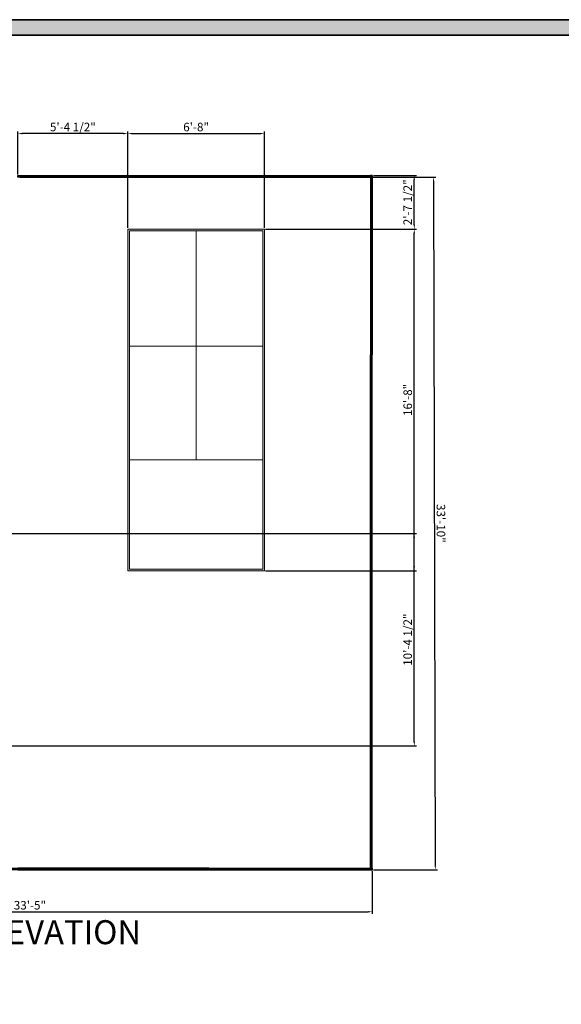
# Model space of a CAD drawing. Units: inches. Extents: x 1804 to 3296, y 909 to 2477.
# Tile 28 of 31: x 2117 to 2434, y 1900 to 2477. Entities that reach past the tile are written whole.
import ezdxf

# ---------------------------------------------------------------- set-up
doc = ezdxf.new("R2010")
doc.units = ezdxf.units.IN
for name, color, linetype, lineweight in [('A-ANNO-DIMS', 2, 'Continuous', 18), ('A-ANNO-TTLB', 156, 'Continuous', 35), ('A-ELEV-PATT', 85, 'Continuous', 13), ('A-WALL-PATT', 10, 'Continuous', 13), ('ELE', 210, 'Continuous', 30), ('TEXT', 190, 'Continuous', 18), ('WIND', 130, 'Continuous', 18)]:
    doc.layers.add(name, color=color, linetype=linetype, lineweight=lineweight)
doc.styles.get("Standard").update_dxf_attribs({"font": 'arial.ttf'})
doc.dimstyles.new('ISO-25', dxfattribs={"dimtxt": 5, "dimasz": 2.5, "dimexe": 1.25, "dimexo": 0.625, "dimtad": 1, "dimdec": 0, "dimlunit": 4, "dimtxsty": 'Standard', "dimcen": 2.5, "dimadec": 0, "dimazin": 0, "dimtfac": 1, "dimtdec": 0, "dimtmove": 0, "dimatfit": 3, "dimfxl": 1, "dimarcsym": 0})

# ---------------------------------------------------------------- blocks, each defined once
blk = doc.blocks.new('*D32')
at = {"layer": 'A-ANNO-DIMS', "color": 0, "lineweight": -2, "transparency": 16777216}
for p, q in [((2322.75, 2384.31), (2360.22, 2384.4)), ((2358.98, 2381.9), (2359.97, 1981.38)), ((2323.75, 1978.79), (2361.22, 1978.88))]:
    blk.add_line(p, q, dxfattribs=at)
at = {"layer": 'A-ANNO-DIMS', "color": 0, "lineweight": 100, "transparency": 16777216}
for points in [[(2359.4, 2381.9), (2358.56, 2381.9), (2358.97, 2384.4)], [(2360.38, 1981.38), (2359.55, 1981.38), (2359.97, 1978.88)]]:
    blk.add_solid(points, dxfattribs=at)
at = {"layer": 'Defpoints', "color": 0, "lineweight": 100, "transparency": 16777216}
for p in [(2322.12, 2384.31), (2323.12, 1978.79), (2359.97, 1978.88)]:
    blk.add_point(p, dxfattribs=at)
at = {"layer": 'A-ANNO-DIMS', "color": 0, "transparency": 16777216, "insert": (2362.65, 2181.65), "char_height": 5, "attachment_point": 5, "rotation": 270.14129}
blk.add_mtext('33\'-10"', dxfattribs=at)
blk = doc.blocks.new('*D75')
at = {"layer": 'A-ANNO-DIMS', "color": 0, "lineweight": -2, "transparency": 16777216}
for p, q in [((1922.17, 1978.16), (1922.17, 1952.99)), ((2323.12, 1978.16), (2323.12, 1952.99)), ((1924.67, 1954.24), (2320.62, 1954.24))]:
    blk.add_line(p, q, dxfattribs=at)
at = {"layer": 'A-ANNO-DIMS', "color": 0, "lineweight": 100, "transparency": 16777216}
for points in [[(1924.67, 1954.65), (1924.67, 1953.82), (1922.17, 1954.24)], [(2320.62, 1954.65), (2320.62, 1953.82), (2323.12, 1954.24)]]:
    blk.add_solid(points, dxfattribs=at)
at = {"layer": 'Defpoints', "color": 0, "lineweight": 100, "transparency": 16777216}
for p in [(1922.17, 1978.79), (2323.12, 1978.79), (2323.12, 1954.24)]:
    blk.add_point(p, dxfattribs=at)
at = {"layer": 'A-ANNO-DIMS', "color": 0, "transparency": 16777216, "insert": (2122.65, 1957.42), "char_height": 5, "attachment_point": 5}
blk.add_mtext('33\'-5"', dxfattribs=at)
blk = doc.blocks.new('*D83')
at = {"layer": 'A-ANNO-DIMS', "color": 0, "lineweight": -2, "transparency": 16777216}
for p, q in [((2054.05, 2175.81), (2348.92, 2175.81)), ((2347.67, 2053.81), (2347.67, 2173.31)), ((2054.05, 2051.31), (2348.92, 2051.31))]:
    blk.add_line(p, q, dxfattribs=at)
at = {"layer": 'A-ANNO-DIMS', "color": 0, "lineweight": 100, "transparency": 16777216}
for points in [[(2347.26, 2173.31), (2348.09, 2173.31), (2347.67, 2175.81)], [(2347.26, 2053.81), (2348.09, 2053.81), (2347.67, 2051.31)]]:
    blk.add_solid(points, dxfattribs=at)
at = {"layer": 'Defpoints', "color": 0, "lineweight": 100, "transparency": 16777216}
for p in [(2053.42, 2175.81), (2347.67, 2175.81), (2053.42, 2051.31)]:
    blk.add_point(p, dxfattribs=at)
at = {"layer": 'A-ANNO-DIMS', "color": 0, "transparency": 16777216, "insert": (2344.46, 2113.56), "char_height": 5, "attachment_point": 5, "rotation": 90}
blk.add_mtext('10\'-4 1/2"', dxfattribs=at)
blk = doc.blocks.new('*D84')
at = {"layer": 'A-ANNO-DIMS', "color": 0, "lineweight": -2, "transparency": 16777216}
for p, q in [((2179.93, 2354.6), (2179.93, 2411.11)), ((2182.43, 2409.86), (2257.48, 2409.86)), ((2259.98, 2354.6), (2259.98, 2411.11))]:
    blk.add_line(p, q, dxfattribs=at)
at = {"layer": 'A-ANNO-DIMS', "color": 0, "lineweight": 100, "transparency": 16777216}
for points in [[(2182.43, 2410.28), (2182.43, 2409.44), (2179.93, 2409.86)], [(2257.48, 2410.28), (2257.48, 2409.44), (2259.98, 2409.86)]]:
    blk.add_solid(points, dxfattribs=at)
at = {"layer": 'Defpoints', "color": 0, "lineweight": 100, "transparency": 16777216}
for p in [(2259.98, 2409.86), (2179.93, 2353.97), (2259.98, 2353.97)]:
    blk.add_point(p, dxfattribs=at)
at = {"layer": 'A-ANNO-DIMS', "color": 0, "transparency": 16777216, "insert": (2219.96, 2413.04), "char_height": 5, "attachment_point": 5}
blk.add_mtext('6\'-8"', dxfattribs=at)
blk = doc.blocks.new('*D85')
at = {"layer": 'A-ANNO-DIMS', "color": 0, "lineweight": -2, "transparency": 16777216}
for p, q in [((2260.61, 2353.97), (2348.92, 2353.97)), ((2347.67, 2156.42), (2347.67, 2351.47)), ((2260.61, 2153.92), (2348.92, 2153.92))]:
    blk.add_line(p, q, dxfattribs=at)
at = {"layer": 'A-ANNO-DIMS', "color": 0, "lineweight": 100, "transparency": 16777216}
for points in [[(2347.26, 2351.47), (2348.09, 2351.47), (2347.67, 2353.97)], [(2347.26, 2156.42), (2348.09, 2156.42), (2347.67, 2153.92)]]:
    blk.add_solid(points, dxfattribs=at)
at = {"layer": 'Defpoints', "color": 0, "lineweight": 100, "transparency": 16777216}
for p in [(2259.98, 2353.97), (2347.67, 2353.97), (2259.98, 2153.92)]:
    blk.add_point(p, dxfattribs=at)
at = {"layer": 'A-ANNO-DIMS', "color": 0, "transparency": 16777216, "insert": (2344.5, 2253.94), "char_height": 5, "attachment_point": 5, "rotation": 90}
blk.add_mtext('16\'-8"', dxfattribs=at)
blk = doc.blocks.new('*D86')
at = {"layer": 'A-ANNO-DIMS', "color": 0, "lineweight": -2, "transparency": 16777216}
for p, q in [((2115.67, 2385.93), (2115.67, 2411.11)), ((2177.43, 2409.86), (2118.17, 2409.86)), ((2179.93, 2354.6), (2179.93, 2411.11))]:
    blk.add_line(p, q, dxfattribs=at)
at = {"layer": 'A-ANNO-DIMS', "color": 0, "lineweight": 100, "transparency": 16777216}
for points in [[(2118.17, 2410.28), (2118.17, 2409.44), (2115.67, 2409.86)], [(2177.43, 2410.28), (2177.43, 2409.44), (2179.93, 2409.86)]]:
    blk.add_solid(points, dxfattribs=at)
at = {"layer": 'Defpoints', "color": 0, "lineweight": 100, "transparency": 16777216}
for p in [(2115.67, 2409.86), (2115.67, 2385.31), (2179.93, 2353.97)]:
    blk.add_point(p, dxfattribs=at)
at = {"layer": 'A-ANNO-DIMS', "color": 0, "transparency": 16777216, "insert": (2147.8, 2413.07), "char_height": 5, "attachment_point": 5}
blk.add_mtext('5\'-4 1/2"', dxfattribs=at)
blk = doc.blocks.new('*D87')
at = {"layer": 'A-ANNO-DIMS', "color": 0, "lineweight": -2, "transparency": 16777216}
for p, q in [((2323.75, 2385.31), (2348.92, 2385.31)), ((2347.67, 2356.47), (2347.67, 2382.81)), ((2260.61, 2353.97), (2348.92, 2353.97))]:
    blk.add_line(p, q, dxfattribs=at)
at = {"layer": 'A-ANNO-DIMS', "color": 0, "lineweight": 100, "transparency": 16777216}
for points in [[(2347.26, 2382.81), (2348.09, 2382.81), (2347.67, 2385.31)], [(2347.26, 2356.47), (2348.09, 2356.47), (2347.67, 2353.97)]]:
    blk.add_solid(points, dxfattribs=at)
at = {"layer": 'Defpoints', "color": 0, "lineweight": 100, "transparency": 16777216}
for p in [(2323.12, 2385.31), (2347.67, 2385.31), (2259.98, 2353.97)]:
    blk.add_point(p, dxfattribs=at)
at = {"layer": 'A-ANNO-DIMS', "color": 0, "transparency": 16777216, "insert": (2344.46, 2369.64), "char_height": 5, "attachment_point": 5, "rotation": 90}
blk.add_mtext('2\'-7 1/2"', dxfattribs=at)

msp = doc.modelspace()

# ---------------------------------------------------------------- hatches: boundary and pattern name
at = {"layer": 'A-ANNO-TTLB'}
h = msp.add_hatch(color=256, dxfattribs=at)
h.dxf.hatch_style = 1
h.paths.add_polyline_path([(3294.53, 2476.54), (1803.79, 2476.54), (1805.43, 909.47), (3296.17, 909.47)])
h.paths.add_polyline_path([(1811, 914.33), (1812.79, 2467.54), (3285.53, 2467.54), (3283.74, 914.33)], flags=16)
h.paths.add_polyline_path([(1925.58, 1062.77), (1925.58, 1138.07), (1925.58, 1539.88), (1925.58, 1793.38), (1925.58, 1830.04), (2325.54, 1830.04), (2325.54, 1793.38), (2325.54, 1586.42), (2325.54, 1138.07), (2325.54, 1062.77)], flags=0)
h.paths.add_polyline_path([(1997.22, 1029.4), (2008.85, 1037.96), (2008.85, 1020.84)], flags=0)
h.paths.add_polyline_path([(1934.58, 1138.07), (1934.58, 1147.07), (2078.77, 1147.07), (2078.77, 1138.07), (2060.94, 1138.07)], flags=0)
h.paths.add_polyline_path([(1944.35, 1138.07), (1944.35, 1147.07), (2056.05, 1147.07), (2056.05, 1138.07)], flags=0)
h.paths.add_polyline_path([(2222.24, 1037.96), (2233.87, 1029.4), (2222.24, 1020.84)], flags=0)
h.paths.add_polyline_path([(2061.94, 1139.07), (2061.94, 1146.07), (2077.77, 1146.07), (2077.77, 1139.07)], flags=0)
h.paths.add_polyline_path([(2149.58, 1138.07), (2149.58, 1269.44), (2158.58, 1269.44), (2158.58, 1326.69), (2149.58, 1326.69), (2149.58, 1340.94), (2139.6, 1340.94), (2139.6, 1434.25), (2149.58, 1434.25), (2149.58, 1447.36), (2158.58, 1447.36), (2158.58, 1423.87), (2158.58, 1408.06), (2198.46, 1408.06), (2198.46, 1412.56), (2282.65, 1412.56), (2282.65, 1465.94), (2316.54, 1465.94), (2316.54, 1590.92), (2192.86, 1590.92), (2192.86, 1595.3), (2291.17, 1595.3), (2291.17, 1590.92), (2316.54, 1590.92), (2316.54, 1784.38), (2300.24, 1784.38), (2300.24, 1757.47), (2268, 1757.47), (2268, 1681.04), (2180.87, 1681.04), (2180.87, 1757.47), (2148.63, 1757.47), (2148.63, 1784.38), (2119.08, 1784.38), (2119.08, 1585.58), (2114.58, 1585.58), (2114.58, 1784.38), (2064.11, 1784.38), (2046.28, 1784.38), (2046.28, 1760.38), (1958.58, 1760.38), (1958.58, 1664.38), (1934.58, 1664.38), (1934.58, 1784.38), (1934.58, 1793.38), (2046.28, 1793.38), (2064.11, 1793.38), (2119.08, 1793.38), (2230.78, 1793.38), (2230.78, 1784.38), (2268, 1784.38), (2300.24, 1784.38), (2316.54, 1784.38), (2316.54, 1590.92), (2316.54, 1373.73), (2316.54, 1138.07)], flags=0)
h.paths.add_polyline_path([(2209.19, 1166.63), (2209.19, 1175.63), (2158.58, 1175.63), (2209.19, 1223.63), (2209.19, 1231.63), (2183.88, 1231.63), (2183.88, 1301.66), (2242.59, 1301.66), (2242.59, 1326.69), (2316.54, 1326.69), (2272.59, 1271.63), (2272.59, 1223.63), (2316.54, 1175.63), (2272.59, 1175.63), (2272.59, 1166.63)], flags=0)
h.paths.add_polyline_path([(1947.77, 1345.22), (1947.77, 1457.48), (1991.2, 1457.48), (1991.2, 1451.7), (1991.2, 1352.18), (1991.2, 1345.22)], flags=0)
h.paths.add_polyline_path([(2209.19, 1271.63), (2262.59, 1271.63), (2262.59, 1311.85), (2272.59, 1301.66), (2272.59, 1271.63), (2269.92, 1269.63), (2270.59, 1269.63), (2270.59, 1225.63), (2211.19, 1225.63), (2211.19, 1269.63), (2211.86, 1269.63)], flags=0)
h.paths.add_polyline_path([(2000.34, 1378.21), (2000.34, 1429.71), (2025.22, 1429.71), (2025.22, 1378.21)], flags=0)
h.paths.add_polyline_path([(2001.34, 1379.21), (2001.34, 1428.71), (2024.22, 1428.71), (2024.22, 1379.21)], flags=0)
h.paths.add_polyline_path([(2012.34, 1390.21), (2012.34, 1417.71), (2013.22, 1417.71), (2013.22, 1390.21)], flags=0)
h.paths.add_polyline_path([(2237.56, 1331.19), (2237.56, 1340.18), (2238.62, 1340.18), (2238.62, 1386.84), (2241.04, 1386.84), (2242.06, 1386.84), (2242.06, 1408.06), (2316.54, 1331.19)], flags=0)
h.paths.add_polyline_path([(1953.73, 1464.35), (1953.73, 1498.59), (1981.74, 1498.59), (1981.74, 1464.35)], flags=0)
h.paths.add_polyline_path([(1987.63, 1462.08), (1987.63, 1500.95), (2104.07, 1500.95), (2104.07, 1462.08), (2099.27, 1462.08), (1993.6, 1462.08)], flags=0)
h.paths.add_polyline_path([(1956.06, 1481.47, -1), (1979.41, 1481.47, -1)], flags=0)
edge = h.paths.add_edge_path(flags=0)
edge.add_ellipse((2299.53, 1438.37), major_axis=(0.31, 21.36), ratio=0.670333, start_angle=0, end_angle=360)
h.paths.add_polyline_path([(2297.39, 1438.37, -1), (2301.67, 1438.37, -1)], flags=0)
h.paths.add_polyline_path([(2591.54, 1163.23), (2591.54, 1179.38), (2591.54, 1379.68), (2591.54, 1395.84), (2734.5, 1395.84), (2734.5, 1379.68), (2734.5, 1179.38), (2734.5, 1163.23)], flags=0)
h.paths.add_polyline_path([(2592.54, 1164.23), (2592.54, 1166.23), (2733.5, 1166.23), (2733.5, 1164.23)], flags=0)
h.paths.add_polyline_path([(2592.54, 1180.38), (2592.54, 1378.68), (2733.5, 1378.68), (2733.5, 1180.38)], flags=0)
h.paths.add_polyline_path([(2593.54, 1181.38), (2593.54, 1377.68), (2732.5, 1377.68), (2732.5, 1181.38)], flags=0)
h.paths.add_polyline_path([(2594.54, 1182.38), (2594.54, 1376.68), (2731.5, 1376.68), (2731.5, 1182.38)], flags=0)
h.paths.add_polyline_path([(1936.95, 1697.46), (1936.95, 1736.46), (1955.41, 1736.46), (1955.41, 1697.46)], flags=0)
h.paths.add_polyline_path([(1938.48, 1718.36), (1938.48, 1734.92), (1953.65, 1734.92), (1953.65, 1718.36)], flags=0)
h.paths.add_polyline_path([(1944.75, 1726.64, -1), (1947.37, 1726.64, -1)], flags=0)
h.paths.add_polyline_path([(2592.54, 1394.84), (2733.5, 1394.84), (2733.5, 1392.84), (2592.54, 1392.84)], flags=0)
h.paths.add_polyline_path([(1976.61, 1762.5), (1976.61, 1781.44), (2012.79, 1781.44), (2012.79, 1762.5)], flags=0)
h.paths.add_polyline_path([(1979.57, 1771.97, -1), (1991.39, 1771.97, -1)], flags=0)
h.paths.add_polyline_path([(1995.36, 1771.97, -1), (2007.18, 1771.97, -1)], flags=0)
h.paths.add_polyline_path([(2251.51, 1744.53), (2268, 1730.05), (2251.51, 1730.05)], flags=0)
h.paths.add_polyline_path([(2047.28, 1785.38), (2047.28, 1792.38), (2063.11, 1792.38), (2063.11, 1785.38)], flags=0)
h.paths.add_polyline_path([(2155.08, 1770.92, -1), (2174.42, 1770.92, -1)], flags=0)
h.paths.add_polyline_path([(2188.59, 1758.27), (2188.59, 1772.81), (2222.3, 1772.81), (2222.3, 1758.27)], flags=0)
h.paths.add_polyline_path([(2223.97, 1758.27), (2223.97, 1772.81), (2257.68, 1772.81), (2257.68, 1758.27)], flags=0)
h.paths.add_polyline_path([(2274.45, 1770.92, -1), (2293.8, 1770.92, -1)], flags=0)
h.paths.add_polyline_path([(2591.54, 1582.09), (2591.54, 1782.39), (2734.5, 1782.39), (2734.5, 1582.09)], flags=0)
h.paths.add_polyline_path([(2592.54, 1583.09), (2592.54, 1781.39), (2733.5, 1781.39), (2733.5, 1583.09)], flags=0)
h.paths.add_polyline_path([(2593.54, 1584.09), (2593.54, 1780.39), (2732.5, 1780.39), (2732.5, 1584.09)], flags=0)
h.paths.add_polyline_path([(2594.54, 1585.09), (2594.54, 1779.39), (2731.5, 1779.39), (2731.5, 1585.09)], flags=0)
h.paths.add_polyline_path([(1922.17, 1978.79), (1922.17, 2295.08), (1922.17, 2296.08), (2115.67, 2296.08), (2115.67, 2384.31), (2115.67, 2385.31), (2322.12, 2385.31), (2323.12, 2385.31), (2323.12, 1979.79), (2323.12, 1978.79), (1923.17, 1978.79)], flags=0)
h.paths.add_polyline_path([(1922.17, 1978.79), (1922.17, 2051.31), (1922.17, 2214.86), (1922.17, 2296.08), (2115.67, 2296.08), (2115.67, 2385.31), (2323.12, 2385.31), (2323.12, 2280.42), (2323.12, 1978.79), (2115.67, 1978.79)], flags=0)
h.paths.add_polyline_path([(1923.17, 1979.79), (1923.17, 2050.31), (2115.67, 2050.31), (2115.67, 2051.31), (1923.17, 2051.31), (1923.17, 2213.86), (1923.17, 2214.86), (1923.17, 2295.08), (1990.02, 2295.08), (1990.02, 2214.86), (1991.02, 2214.86), (1991.02, 2295.08), (2115.67, 2295.08), (2115.67, 1979.79), (2116.67, 1979.79), (2116.67, 2304.18), (2116.67, 2384.31), (2322.12, 2384.31), (2322.12, 2280.42), (2322.12, 1979.79), (2115.67, 1979.79)], flags=0)
h.paths.add_polyline_path([(2972.46, 1192.5), (2972.46, 1196.92), (2995.47, 1196.92), (2995.47, 1255.47), (2995.09, 1255.47), (2987.42, 1249.39), (2980.08, 1255.47), (2978.05, 1255.47), (2978.05, 1257.24), (2995.47, 1257.24), (2995.47, 1261.58), (3015.37, 1261.58), (3015.37, 1333.28), (3015.37, 1414.4), (3032.82, 1414.4), (3032.82, 1333.28), (3032.82, 1261.58), (3052.66, 1261.58), (3052.66, 1255.47), (3079.86, 1255.47), (3078.72, 1254.57), (3081.47, 1252.29), (3078.56, 1249.99), (3075.81, 1252.26), (3072.57, 1249.69), (3070.36, 1251.52), (3067.67, 1249.39), (3060.34, 1255.47), (3052.66, 1255.47), (3052.66, 1196.92), (3054.58, 1196.92), (3074, 1196.92), (3074, 1192.5), (3052.66, 1192.5), (2995.47, 1192.5)], flags=0)
h.paths.add_polyline_path([(2490.75, 1979.27), (2490.75, 1980.27), (2596.87, 1980.27), (2596.87, 2051.8), (2596.87, 2052.8), (2596.87, 2216.35), (2596.87, 2297.57), (2717.32, 2297.57), (2710.57, 2305.62), (2724.07, 2305.62), (2717.32, 2297.57), (2782.37, 2297.57), (2782.37, 2395.8), (3006.82, 2395.8), (3006.82, 1981.27), (3093.73, 1981.27), (3093.73, 1980.27), (3047.51, 1980.27), (3046.37, 1979.37), (3049.11, 1977.1), (3046.2, 1974.79), (3043.46, 1977.07), (3040.21, 1974.49), (3038, 1976.32), (3035.32, 1974.2), (3027.98, 1980.27), (2871.83, 1980.27), (2871.83, 1981.27), (2791.37, 1981.27), (2791.37, 2050.8), (2597.87, 2050.8), (2597.87, 1980.27), (2597.87, 1979.27), (2546.27, 1979.27), (2545.12, 1978.37), (2547.87, 1976.1), (2544.96, 1973.79), (2542.22, 1976.07), (2538.97, 1973.49), (2536.76, 1975.32), (2534.07, 1973.2), (2526.74, 1979.27)], flags=0)
h.paths.add_polyline_path([(2597.87, 2051.8), (2606.87, 2051.8), (2606.87, 2258.39), (2597.87, 2258.39), (2597.87, 2296.57), (2606.87, 2296.57), (2606.87, 2262.39), (2782.37, 2262.39), (2782.37, 2296.57), (2790.37, 2296.57), (2790.37, 2262.39), (2791.37, 2262.39), (2791.37, 2305.67), (2791.37, 2385.8), (2996.82, 2385.8), (2996.82, 2339.85), (3006.82, 2339.85), (3006.82, 2250.12), (2997.82, 2250.12), (2997.82, 1981.27), (2996.82, 1981.27), (2872.83, 1981.27), (2872.83, 1991.8), (2871.83, 1991.8), (2871.83, 2050.8), (2790.37, 2050.8), (2597.87, 2050.8)], flags=0)
h.paths.add_polyline_path([(2179.93, 2153.92), (2179.93, 2353.97), (2259.98, 2353.97), (2259.98, 2153.92)], flags=0)
h.paths.add_polyline_path([(2180.93, 2154.92), (2180.93, 2352.97), (2258.98, 2352.97), (2258.98, 2154.92)], flags=0)
h.paths.add_polyline_path([(2960.87, 1608.49), (2960.87, 1753.62), (3070.9, 1753.62), (3070.9, 1608.49)], flags=0)
h.paths.add_polyline_path([(2961.87, 1609.49), (2961.87, 1752.62), (3069.9, 1752.62), (3069.9, 1609.49)], flags=0)
h.paths.add_polyline_path([(2962.87, 1610.49), (2962.87, 1751.62), (3068.9, 1751.62), (3068.9, 1610.49)], flags=0)
h.paths.add_polyline_path([(2963.87, 1611.49), (2963.87, 1750.62), (3067.9, 1750.62), (3067.9, 1611.49)], flags=0)
h.paths.add_polyline_path([(2782.37, 2051.8), (2782.37, 2216.32), (2791.37, 2216.32), (2791.37, 2051.8), (2872.83, 2051.8), (2872.83, 2068.56), (2884.67, 2068.56), (2884.67, 2085.33), (2896.51, 2085.33), (2896.51, 2102.09), (2908.36, 2102.09), (2908.36, 2118.85), (2920.2, 2118.85), (2920.2, 2135.62), (2932.05, 2135.62), (2932.05, 2145.3), (2925.08, 2145.3), (2925.08, 2203.2), (2996.82, 2203.2), (2996.82, 2145.3), (2953.82, 2145.3), (2872.83, 2051.8), (2790.37, 2051.8)], flags=0)
h.paths.add_polyline_path([(2717.32, 2238.65), (2710.57, 2246.7), (2724.07, 2246.7)], flags=0)
h.paths.add_polyline_path([(2003.09, 1122.79), (2017.16, 1122.79), (2017.16, 1138.74), (2003.09, 1138.74)], flags=8)
h.paths.add_polyline_path([(2174.76, 1792.72), (2188.83, 1792.72), (2188.83, 1808.66), (2174.76, 1808.66)], flags=8)
h.paths.add_polyline_path([(1987.95, 1792.51), (2002.02, 1792.51), (2002.02, 1808.45), (1987.95, 1808.45)], flags=8)
h.paths.add_polyline_path([(2148.79, 1289.26), (2160.46, 1289.26), (2160.46, 1305.2), (2148.79, 1305.2)], flags=8)
h.paths.add_polyline_path([(2115.36, 1133.57), (2127.04, 1133.57), (2127.04, 1149.51), (2115.36, 1149.51)], flags=8)
h.paths.add_polyline_path([(2237.58, 1421.48), (2249.25, 1421.48), (2249.25, 1437.43), (2237.58, 1437.43)], flags=8)
h.paths.add_polyline_path([(2134.99, 1584.32), (2146.66, 1584.32), (2146.66, 1600.26), (2134.99, 1600.26)], flags=8)
h.paths.add_polyline_path([(2101.95, 1557.31), (2113.62, 1557.31), (2113.62, 1573.25), (2101.95, 1573.25)], flags=8)
h.paths.add_polyline_path([(2937.85, 1156.77), (3120.41, 1156.77), (3120.41, 1185.72), (2937.85, 1185.72)], flags=8)
h.paths.add_polyline_path([(2980.71, 1786.71), (3050.06, 1786.71), (3050.06, 1802.66), (2980.71, 1802.66)], flags=8)
h.paths.add_polyline_path([(2869.28, 1661.96), (2938.62, 1661.96), (2938.62, 1690.8), (2869.28, 1690.8)], flags=8)
h.paths.add_polyline_path([(3092.27, 1674.86), (3161.62, 1674.86), (3161.62, 1690.8), (3092.27, 1690.8)], flags=8)
h.paths.add_polyline_path([(2980.71, 1674.86), (3050.06, 1674.86), (3050.06, 1690.8), (2980.71, 1690.8)], flags=8)
h.paths.add_polyline_path([(2649.07, 1678.23), (2674.53, 1678.23), (2674.53, 1714.76), (2649.07, 1714.76)], flags=8)
h.paths.add_polyline_path([(2530.84, 1981.63), (2549.13, 1981.63), (2549.13, 1997.57), (2530.84, 1997.57)], flags=8)
h.paths.add_polyline_path([(3031.29, 1981.77), (3049.58, 1981.77), (3049.58, 1997.71), (3031.29, 1997.71)], flags=8)
h.paths.add_polyline_path([(2715.38, 1911.9), (2851.54, 1911.9), (2851.54, 1940.85), (2715.38, 1940.85)], flags=8)
h.paths.add_polyline_path([(2015.23, 1927.36), (2205.42, 1927.36), (2205.42, 1956.3), (2015.23, 1956.3)], flags=8)
h.paths.add_polyline_path([(2671.84, 2057.84), (2702.75, 2057.84), (2702.75, 2073.79), (2671.84, 2073.79)], flags=8)
h.paths.add_polyline_path([(2678.5, 2316.52), (2765.26, 2316.52), (2765.26, 2332.46), (2678.5, 2332.46)], flags=8)
h.paths.add_polyline_path([(2678.48, 2271.96), (2736.41, 2271.96), (2736.41, 2287.9), (2678.48, 2287.9)], flags=8)
h.paths.add_polyline_path([(2019.2, 972.79), (2243.21, 972.79), (2243.21, 1001.74), (2019.2, 1001.74)], flags=8)
h.paths.add_polyline_path([(2097.06, 1021.56), (2132.16, 1021.56), (2132.16, 1037.51), (2097.06, 1037.51)], flags=8)
h.paths.add_polyline_path([(2182.47, 1360.48), (2207.35, 1360.48), (2207.35, 1376.42), (2182.47, 1376.42)], flags=8)
h.paths.add_polyline_path([(2261.12, 1361.77), (2295.01, 1361.77), (2295.01, 1377.71), (2261.12, 1377.71)], flags=8)
h.paths.add_polyline_path([(2245.75, 1511.51), (2278.44, 1511.51), (2278.44, 1527.46), (2245.75, 1527.46)], flags=8)
h.paths.add_polyline_path([(1991.16, 1296.29), (2060.51, 1296.29), (2060.51, 1312.23), (1991.16, 1312.23)], flags=8)
h.paths.add_polyline_path([(2187, 1651.35), (2246.71, 1651.35), (2246.71, 1667.29), (2187, 1667.29)], flags=8)
h.paths.add_polyline_path([(1976.49, 1684.81), (2068.63, 1684.81), (2068.63, 1700.76), (1976.49, 1700.76)], flags=8)
at = {"layer": 'A-ELEV-PATT'}
h = msp.add_hatch(color=256, dxfattribs=at)
h.dxf.hatch_style = 1
h.paths.add_polyline_path([(2322.12, 2385.31), (2115.67, 2385.31), (2115.67, 2384.31), (2322.12, 2384.31)])
h = msp.add_hatch(color=256, dxfattribs=at)
h.dxf.hatch_style = 1
h.paths.add_polyline_path([(2323.12, 2385.31), (2322.12, 2385.31), (2322.12, 1979.79), (2323.12, 1979.79)])
h = msp.add_hatch(color=256, dxfattribs=at)
h.dxf.hatch_style = 1
h.paths.add_polyline_path([(2179.93, 2153.92), (2259.98, 2153.92), (2259.98, 2353.97), (2179.93, 2353.97)])
h.paths.add_polyline_path([(2180.93, 2154.92), (2258.98, 2154.92), (2258.98, 2352.97), (2180.93, 2352.97)], flags=16)
h = msp.add_hatch(color=256, dxfattribs=at)
h.dxf.hatch_style = 1
h.paths.add_polyline_path([(2323.12, 1979.79), (1923.17, 1979.79), (1923.17, 1978.79), (2323.12, 1978.79)])
at = {"layer": 'A-WALL-PATT'}
h = msp.add_hatch(color=256, dxfattribs=at)
h.dxf.hatch_style = 1
h.paths.add_polyline_path([(2119.08, 1544.38), (1925.58, 1544.38), (1925.58, 1539.88), (2119.08, 1539.88)])
h.paths.add_polyline_path([(2119.08, 1545.58), (2114.58, 1545.58), (2114.58, 1544.38), (2119.08, 1544.38)])
h.paths.add_polyline_path([(1965.87, 1658.79), (1965.87, 1679.09), (1955.57, 1679.09), (1955.57, 1658.79)], flags=9)
h.paths.add_polyline_path([(2293.18, 1677.29), (2293.18, 1697.58), (2282.88, 1697.58), (2282.88, 1677.29)], flags=9)
h.paths.add_polyline_path([(2271.13, 1545.23), (2287.53, 1545.23), (2287.53, 1555.53), (2271.13, 1555.53)], flags=9)
h.paths.add_polyline_path([(2303.26, 1488.52), (2303.26, 1508.82), (2292.95, 1508.82), (2292.95, 1488.52)], flags=9)
h.paths.add_polyline_path([(2271.13, 1393.15), (2287.53, 1393.15), (2287.53, 1403.45), (2271.13, 1403.45)], flags=9)
h.paths.add_polyline_path([(2306.48, 1361.45), (2306.48, 1377.86), (2296.18, 1377.86), (2296.18, 1361.45)], flags=9)
h.paths.add_polyline_path([(2174.54, 1361.45), (2174.54, 1377.86), (2164.23, 1377.86), (2164.23, 1361.45)], flags=9)
h.paths.add_polyline_path([(1968.21, 1333.34), (1968.21, 1353.64), (1957.91, 1353.64), (1957.91, 1333.34)], flags=9)
h.paths.add_polyline_path([(2003.09, 1122.79), (2017.16, 1122.79), (2017.16, 1138.74), (2003.09, 1138.74)], flags=9)
h.paths.add_polyline_path([(2174.76, 1792.72), (2188.83, 1792.72), (2188.83, 1808.66), (2174.76, 1808.66)], flags=9)
h.paths.add_polyline_path([(1987.95, 1792.51), (2002.02, 1792.51), (2002.02, 1808.45), (1987.95, 1808.45)], flags=9)
h.paths.add_polyline_path([(2148.79, 1289.26), (2160.46, 1289.26), (2160.46, 1305.2), (2148.79, 1305.2)], flags=9)
h.paths.add_polyline_path([(2115.36, 1133.57), (2127.04, 1133.57), (2127.04, 1149.51), (2115.36, 1149.51)], flags=9)
h.paths.add_polyline_path([(2237.58, 1421.48), (2249.25, 1421.48), (2249.25, 1437.43), (2237.58, 1437.43)], flags=9)
h.paths.add_polyline_path([(2134.99, 1584.32), (2146.66, 1584.32), (2146.66, 1600.26), (2134.99, 1600.26)], flags=9)
h.paths.add_polyline_path([(2101.95, 1557.31), (2113.62, 1557.31), (2113.62, 1573.25), (2101.95, 1573.25)], flags=9)
h.paths.add_polyline_path([(2937.85, 1156.77), (3120.41, 1156.77), (3120.41, 1185.72), (2937.85, 1185.72)], flags=9)
h.paths.add_polyline_path([(2980.71, 1786.71), (3050.06, 1786.71), (3050.06, 1802.66), (2980.71, 1802.66)], flags=9)
h.paths.add_polyline_path([(2869.28, 1661.96), (2938.62, 1661.96), (2938.62, 1690.8), (2869.28, 1690.8)], flags=9)
h.paths.add_polyline_path([(3092.27, 1674.86), (3161.62, 1674.86), (3161.62, 1690.8), (3092.27, 1690.8)], flags=9)
h.paths.add_polyline_path([(2980.71, 1674.86), (3050.06, 1674.86), (3050.06, 1690.8), (2980.71, 1690.8)], flags=9)
h.paths.add_polyline_path([(2649.07, 1678.23), (2674.53, 1678.23), (2674.53, 1714.76), (2649.07, 1714.76)], flags=9)
h.paths.add_polyline_path([(2530.84, 1981.63), (2549.13, 1981.63), (2549.13, 1997.57), (2530.84, 1997.57)], flags=9)
h.paths.add_polyline_path([(3031.29, 1981.77), (3049.58, 1981.77), (3049.58, 1997.71), (3031.29, 1997.71)], flags=9)
h.paths.add_polyline_path([(2715.38, 1911.9), (2851.54, 1911.9), (2851.54, 1940.85), (2715.38, 1940.85)], flags=9)
h.paths.add_polyline_path([(2015.23, 1927.36), (2205.42, 1927.36), (2205.42, 1956.3), (2015.23, 1956.3)], flags=9)
h.paths.add_polyline_path([(2671.84, 2057.84), (2702.75, 2057.84), (2702.75, 2073.79), (2671.84, 2073.79)], flags=9)
h.paths.add_polyline_path([(2678.5, 2316.52), (2765.26, 2316.52), (2765.26, 2332.46), (2678.5, 2332.46)], flags=9)
h.paths.add_polyline_path([(2678.48, 2271.96), (2736.41, 2271.96), (2736.41, 2287.9), (2678.48, 2287.9)], flags=9)
h.paths.add_polyline_path([(2019.2, 972.79), (2243.21, 972.79), (2243.21, 1001.74), (2019.2, 1001.74)], flags=9)
h.paths.add_polyline_path([(2097.06, 1021.56), (2132.16, 1021.56), (2132.16, 1037.51), (2097.06, 1037.51)], flags=9)
h.paths.add_polyline_path([(2182.47, 1360.48), (2207.35, 1360.48), (2207.35, 1376.42), (2182.47, 1376.42)], flags=9)
h.paths.add_polyline_path([(2261.12, 1361.77), (2295.01, 1361.77), (2295.01, 1377.71), (2261.12, 1377.71)], flags=9)
h.paths.add_polyline_path([(2245.75, 1511.51), (2278.44, 1511.51), (2278.44, 1527.46), (2245.75, 1527.46)], flags=9)
h.paths.add_polyline_path([(1991.16, 1296.29), (2060.51, 1296.29), (2060.51, 1312.23), (1991.16, 1312.23)], flags=9)
h.paths.add_polyline_path([(2187, 1651.35), (2246.71, 1651.35), (2246.71, 1667.29), (2187, 1667.29)], flags=9)
h.paths.add_polyline_path([(1976.49, 1684.81), (2068.63, 1684.81), (2068.63, 1700.76), (1976.49, 1700.76)], flags=9)
h = msp.add_hatch(color=256, dxfattribs=at)
h.dxf.hatch_style = 1
h.paths.add_polyline_path([(2149.58, 1147.07), (2141.21, 1147.07), (2141.21, 1144.07), (2141.21, 1138.07), (2149.58, 1138.07)])
h.paths.add_polyline_path([(2101.21, 1144.07, -0.01877), (2101.32, 1147.07), (2078.77, 1147.07), (2078.77, 1138.07), (2101.21, 1138.07)])
h.paths.add_polyline_path([(2060.94, 1147.07), (2056.05, 1147.07), (2056.05, 1138.07), (2060.94, 1138.07)])
h.paths.add_polyline_path([(1944.35, 1147.07), (1934.58, 1147.07), (1934.58, 1138.07), (1944.35, 1138.07)])
h.paths.add_polyline_path([(2158.58, 1269.44), (2149.58, 1269.44), (2149.58, 1138.07), (2158.58, 1138.07)])
h.paths.add_polyline_path([(2003.09, 1122.79), (2017.16, 1122.79), (2017.16, 1138.74), (2003.09, 1138.74)], flags=9)
h.paths.add_polyline_path([(2174.76, 1792.72), (2188.83, 1792.72), (2188.83, 1808.66), (2174.76, 1808.66)], flags=9)
h.paths.add_polyline_path([(1987.95, 1792.51), (2002.02, 1792.51), (2002.02, 1808.45), (1987.95, 1808.45)], flags=9)
h.paths.add_polyline_path([(2148.79, 1289.26), (2160.46, 1289.26), (2160.46, 1305.2), (2148.79, 1305.2)], flags=9)
h.paths.add_polyline_path([(2115.36, 1133.57), (2127.04, 1133.57), (2127.04, 1149.51), (2115.36, 1149.51)], flags=9)
h.paths.add_polyline_path([(2237.58, 1421.48), (2249.25, 1421.48), (2249.25, 1437.43), (2237.58, 1437.43)], flags=9)
h.paths.add_polyline_path([(2134.99, 1584.32), (2146.66, 1584.32), (2146.66, 1600.26), (2134.99, 1600.26)], flags=9)
h.paths.add_polyline_path([(2101.95, 1557.31), (2113.62, 1557.31), (2113.62, 1573.25), (2101.95, 1573.25)], flags=9)
h.paths.add_polyline_path([(2937.85, 1156.77), (3120.41, 1156.77), (3120.41, 1185.72), (2937.85, 1185.72)], flags=9)
h.paths.add_polyline_path([(2980.71, 1786.71), (3050.06, 1786.71), (3050.06, 1802.66), (2980.71, 1802.66)], flags=9)
h.paths.add_polyline_path([(2869.28, 1661.96), (2938.62, 1661.96), (2938.62, 1690.8), (2869.28, 1690.8)], flags=9)
h.paths.add_polyline_path([(3092.27, 1674.86), (3161.62, 1674.86), (3161.62, 1690.8), (3092.27, 1690.8)], flags=9)
h.paths.add_polyline_path([(2980.71, 1674.86), (3050.06, 1674.86), (3050.06, 1690.8), (2980.71, 1690.8)], flags=9)
h.paths.add_polyline_path([(2649.07, 1678.23), (2674.53, 1678.23), (2674.53, 1714.76), (2649.07, 1714.76)], flags=9)
h.paths.add_polyline_path([(2530.84, 1981.63), (2549.13, 1981.63), (2549.13, 1997.57), (2530.84, 1997.57)], flags=9)
h.paths.add_polyline_path([(3031.29, 1981.77), (3049.58, 1981.77), (3049.58, 1997.71), (3031.29, 1997.71)], flags=9)
h.paths.add_polyline_path([(2715.38, 1911.9), (2851.54, 1911.9), (2851.54, 1940.85), (2715.38, 1940.85)], flags=9)
h.paths.add_polyline_path([(2015.23, 1927.36), (2205.42, 1927.36), (2205.42, 1956.3), (2015.23, 1956.3)], flags=9)
h.paths.add_polyline_path([(2671.84, 2057.84), (2702.75, 2057.84), (2702.75, 2073.79), (2671.84, 2073.79)], flags=9)
h.paths.add_polyline_path([(2678.5, 2316.52), (2765.26, 2316.52), (2765.26, 2332.46), (2678.5, 2332.46)], flags=9)
h.paths.add_polyline_path([(2678.48, 2271.96), (2736.41, 2271.96), (2736.41, 2287.9), (2678.48, 2287.9)], flags=9)
h.paths.add_polyline_path([(2019.2, 972.79), (2243.21, 972.79), (2243.21, 1001.74), (2019.2, 1001.74)], flags=9)
h.paths.add_polyline_path([(2097.06, 1021.56), (2132.16, 1021.56), (2132.16, 1037.51), (2097.06, 1037.51)], flags=9)
h.paths.add_polyline_path([(2182.47, 1360.48), (2207.35, 1360.48), (2207.35, 1376.42), (2182.47, 1376.42)], flags=9)
h.paths.add_polyline_path([(2261.12, 1361.77), (2295.01, 1361.77), (2295.01, 1377.71), (2261.12, 1377.71)], flags=9)
h.paths.add_polyline_path([(2245.75, 1511.51), (2278.44, 1511.51), (2278.44, 1527.46), (2245.75, 1527.46)], flags=9)
h.paths.add_polyline_path([(1991.16, 1296.29), (2060.51, 1296.29), (2060.51, 1312.23), (1991.16, 1312.23)], flags=9)
h.paths.add_polyline_path([(2187, 1651.35), (2246.71, 1651.35), (2246.71, 1667.29), (2187, 1667.29)], flags=9)
h.paths.add_polyline_path([(1976.49, 1684.81), (2068.63, 1684.81), (2068.63, 1700.76), (1976.49, 1700.76)], flags=9)
h = msp.add_hatch(color=256, dxfattribs=at)
h.dxf.hatch_style = 1
h.paths.add_polyline_path([(2158.58, 1275.49), (2155.29, 1275.49), (2149.58, 1275.49), (2149.58, 1269.44), (2158.58, 1269.44)])
h.paths.add_polyline_path([(2158.58, 1326.69), (2149.58, 1326.69), (2149.58, 1319.33), (2155.29, 1319.33), (2158.58, 1319.33)])
h.paths.add_polyline_path([(2158.58, 1402.2), (2158.58, 1423.87), (2158.58, 1447.36), (2149.58, 1447.36), (2149.58, 1423.87), (2149.58, 1340.94), (2149.58, 1326.69), (2158.58, 1326.69), (2158.58, 1354.23)])
h.paths.add_polyline_path([(1965.87, 1658.79), (1965.87, 1679.09), (1955.57, 1679.09), (1955.57, 1658.79)], flags=9)
h.paths.add_polyline_path([(2293.18, 1677.29), (2293.18, 1697.58), (2282.88, 1697.58), (2282.88, 1677.29)], flags=9)
h.paths.add_polyline_path([(2271.13, 1545.23), (2287.53, 1545.23), (2287.53, 1555.53), (2271.13, 1555.53)], flags=9)
h.paths.add_polyline_path([(2303.26, 1488.52), (2303.26, 1508.82), (2292.95, 1508.82), (2292.95, 1488.52)], flags=9)
h.paths.add_polyline_path([(2271.13, 1393.15), (2287.53, 1393.15), (2287.53, 1403.45), (2271.13, 1403.45)], flags=9)
h.paths.add_polyline_path([(2306.48, 1361.45), (2306.48, 1377.86), (2296.18, 1377.86), (2296.18, 1361.45)], flags=9)
h.paths.add_polyline_path([(2189.9, 1340.62), (2206.31, 1340.62), (2206.31, 1350.92), (2189.9, 1350.92)], flags=9)
h.paths.add_polyline_path([(2174.54, 1361.45), (2174.54, 1377.86), (2164.23, 1377.86), (2164.23, 1361.45)], flags=9)
h.paths.add_polyline_path([(2304.24, 1240.8), (2304.24, 1261.09), (2293.94, 1261.09), (2293.94, 1240.8)], flags=9)
h.paths.add_polyline_path([(2227.19, 1188.73), (2247.49, 1188.73), (2247.49, 1199.03), (2227.19, 1199.03)], flags=9)
h.paths.add_polyline_path([(2181.93, 1144.21), (2181.93, 1160.62), (2171.63, 1160.62), (2171.63, 1144.21)], flags=9)
h.paths.add_polyline_path([(1968.21, 1333.34), (1968.21, 1353.64), (1957.91, 1353.64), (1957.91, 1333.34)], flags=9)
h.paths.add_polyline_path([(2029.78, 1203.53), (2053.95, 1203.53), (2053.95, 1213.83), (2029.78, 1213.83)], flags=9)
h.paths.add_polyline_path([(2576.51, 1671.88), (2576.51, 1692.17), (2566.21, 1692.17), (2566.21, 1671.88)], flags=9)
h.paths.add_polyline_path([(2566.99, 1269.67), (2566.99, 1289.96), (2556.68, 1289.96), (2556.68, 1269.67)], flags=9)
h.paths.add_polyline_path([(2581.85, 1269.17), (2581.85, 1289.46), (2571.54, 1289.46), (2571.54, 1269.17)], flags=9)
h.paths.add_polyline_path([(2650.71, 1409.75), (2674.89, 1409.75), (2674.89, 1420.05), (2650.71, 1420.05)], flags=9)
h.paths.add_polyline_path([(2003.09, 1122.79), (2017.16, 1122.79), (2017.16, 1138.74), (2003.09, 1138.74)], flags=9)
h.paths.add_polyline_path([(2174.76, 1792.72), (2188.83, 1792.72), (2188.83, 1808.66), (2174.76, 1808.66)], flags=9)
h.paths.add_polyline_path([(1987.95, 1792.51), (2002.02, 1792.51), (2002.02, 1808.45), (1987.95, 1808.45)], flags=9)
h.paths.add_polyline_path([(2148.79, 1289.26), (2160.46, 1289.26), (2160.46, 1305.2), (2148.79, 1305.2)], flags=9)
h.paths.add_polyline_path([(2115.36, 1133.57), (2127.04, 1133.57), (2127.04, 1149.51), (2115.36, 1149.51)], flags=9)
h.paths.add_polyline_path([(2237.58, 1421.48), (2249.25, 1421.48), (2249.25, 1437.43), (2237.58, 1437.43)], flags=9)
h.paths.add_polyline_path([(2134.99, 1584.32), (2146.66, 1584.32), (2146.66, 1600.26), (2134.99, 1600.26)], flags=9)
h.paths.add_polyline_path([(2101.95, 1557.31), (2113.62, 1557.31), (2113.62, 1573.25), (2101.95, 1573.25)], flags=9)
h.paths.add_polyline_path([(2937.85, 1156.77), (3120.41, 1156.77), (3120.41, 1185.72), (2937.85, 1185.72)], flags=9)
h.paths.add_polyline_path([(2980.71, 1786.71), (3050.06, 1786.71), (3050.06, 1802.66), (2980.71, 1802.66)], flags=9)
h.paths.add_polyline_path([(2869.28, 1661.96), (2938.62, 1661.96), (2938.62, 1690.8), (2869.28, 1690.8)], flags=9)
h.paths.add_polyline_path([(3092.27, 1674.86), (3161.62, 1674.86), (3161.62, 1690.8), (3092.27, 1690.8)], flags=9)
h.paths.add_polyline_path([(2980.71, 1674.86), (3050.06, 1674.86), (3050.06, 1690.8), (2980.71, 1690.8)], flags=9)
h.paths.add_polyline_path([(2649.07, 1678.23), (2674.53, 1678.23), (2674.53, 1714.76), (2649.07, 1714.76)], flags=9)
h.paths.add_polyline_path([(2530.84, 1981.63), (2549.13, 1981.63), (2549.13, 1997.57), (2530.84, 1997.57)], flags=9)
h.paths.add_polyline_path([(3031.29, 1981.77), (3049.58, 1981.77), (3049.58, 1997.71), (3031.29, 1997.71)], flags=9)
h.paths.add_polyline_path([(2715.38, 1911.9), (2851.54, 1911.9), (2851.54, 1940.85), (2715.38, 1940.85)], flags=9)
h.paths.add_polyline_path([(2015.23, 1927.36), (2205.42, 1927.36), (2205.42, 1956.3), (2015.23, 1956.3)], flags=9)
h.paths.add_polyline_path([(2671.84, 2057.84), (2702.75, 2057.84), (2702.75, 2073.79), (2671.84, 2073.79)], flags=9)
h.paths.add_polyline_path([(2678.5, 2316.52), (2765.26, 2316.52), (2765.26, 2332.46), (2678.5, 2332.46)], flags=9)
h.paths.add_polyline_path([(2678.48, 2271.96), (2736.41, 2271.96), (2736.41, 2287.9), (2678.48, 2287.9)], flags=9)
h.paths.add_polyline_path([(2019.2, 972.79), (2243.21, 972.79), (2243.21, 1001.74), (2019.2, 1001.74)], flags=9)
h.paths.add_polyline_path([(2097.06, 1021.56), (2132.16, 1021.56), (2132.16, 1037.51), (2097.06, 1037.51)], flags=9)
h.paths.add_polyline_path([(2182.47, 1360.48), (2207.35, 1360.48), (2207.35, 1376.42), (2182.47, 1376.42)], flags=9)
h.paths.add_polyline_path([(2261.12, 1361.77), (2295.01, 1361.77), (2295.01, 1377.71), (2261.12, 1377.71)], flags=9)
h.paths.add_polyline_path([(2245.75, 1511.51), (2278.44, 1511.51), (2278.44, 1527.46), (2245.75, 1527.46)], flags=9)
h.paths.add_polyline_path([(1991.16, 1296.29), (2060.51, 1296.29), (2060.51, 1312.23), (1991.16, 1312.23)], flags=9)
h.paths.add_polyline_path([(2187, 1651.35), (2246.71, 1651.35), (2246.71, 1667.29), (2187, 1667.29)], flags=9)
h.paths.add_polyline_path([(1976.49, 1684.81), (2068.63, 1684.81), (2068.63, 1700.76), (1976.49, 1700.76)], flags=9)

# ---------------------------------------------------------------- linework, layer by layer
at = {"layer": 'A-ANNO-TTLB'}
for points in [[(1803.79, 2476.54), (3294.53, 2476.54), (3296.17, 909.47), (1805.43, 909.47)], [(1812.79, 2467.54), (3285.53, 2467.54), (3283.74, 914.33), (1811, 914.33)]]:
    msp.add_lwpolyline(points, close=True, dxfattribs=at)
at = {"layer": 'ELE'}
for p, q in [((2115.67, 2385.31), (2323.12, 2385.31)), ((2116.67, 2384.31), (2322.12, 2384.31)), ((2322.12, 2384.31), (2322.12, 2280.42)), ((2323.12, 2385.31), (2323.12, 2280.42)), ((2322.12, 1979.79), (2322.12, 2280.42)), ((2323.12, 1978.79), (2323.12, 2280.42)), ((2115.67, 1979.79), (2322.12, 1979.79)), ((2115.67, 1978.79), (2323.12, 1978.79))]:
    msp.add_line(p, q, dxfattribs=at)
for points in [[(2115.67, 2385.31), (2322.12, 2385.31), (2322.12, 2384.31), (2115.67, 2384.31)], [(2323.12, 2385.31), (2322.12, 2385.31), (2322.12, 1979.79), (2323.12, 1979.79)], [(2323.12, 1978.79), (1923.17, 1978.79), (1923.17, 1979.79), (2323.12, 1979.79)]]:
    msp.add_lwpolyline(points, close=True, dxfattribs=at)
for points in [[(2227.37, 1979.79), (2115.67, 1979.79)], [(2227.37, 1978.79), (2115.67, 1978.79)]]:
    msp.add_lwpolyline(points, dxfattribs=at)
at = {"layer": 'WIND'}
for p, q in [((2219.96, 2218.89), (2219.96, 2352.97)), ((2180.93, 2285.49), (2258.98, 2285.49)), ((2180.93, 2218.89), (2258.98, 2218.89))]:
    msp.add_line(p, q, dxfattribs=at)
for points in [[(2179.93, 2353.97), (2259.98, 2353.97), (2259.98, 2153.92), (2179.93, 2153.92)], [(2180.93, 2352.97), (2258.98, 2352.97), (2258.98, 2154.92), (2180.93, 2154.92)]]:
    msp.add_lwpolyline(points, close=True, dxfattribs=at)

# ---------------------------------------------------------------- texts
at = {"layer": 'TEXT', "insert": (2020.35, 1949.32), "char_height": 14.0468, "attachment_point": 1}
msp.add_mtext_dynamic_manual_height_columns('FRONT ELEVATION', width=296.512, gutter_width=70.23, heights=[0], dxfattribs=at)

# ---------------------------------------------------------------- dimensions: what is measured, and where the dimension line sits
at = {"layer": 'A-ANNO-DIMS'}
for base, p1, p2, picture, middle in [((2115.67, 2409.86), (2179.93, 2353.97), (2115.67, 2385.31), '*D86', (2147.8, 2413.07)), ((2259.9844, 2409.8598), (2179.9258, 2353.9727), (2259.9844, 2353.9727), '*D84', (2219.9551, 2413.0377)), ((2323.1246, 1954.2374), (1922.1699, 1978.7874), (2323.1246, 1978.7874), '*D75', (2122.6473, 1957.417))]:
    dim = msp.add_linear_dim(base=base, p1=p1, p2=p2, dimstyle='ISO-25', override={"dimdec": 1, "dimlfac": 1, "dimrnd": 0, "dimzin": 1, "dimdsep": 46, "dimlunit": 4, "dimfrac": 2}, dxfattribs=at)
    dim.commit()
    dim.dimension.update_dxf_attribs({"geometry": picture, "text_midpoint": middle})
for base, p1, p2, picture, middle in [((2347.67, 2385.31), (2259.98, 2353.97), (2323.12, 2385.31), '*D87', (2344.46, 2369.64)), ((2347.6746, 2353.9727), (2259.9844, 2153.9172), (2259.9844, 2353.9727), '*D85', (2344.4967, 2253.945)), ((2347.67, 2175.81), (2053.42, 2051.31), (2053.42, 2175.81), '*D83', (2344.46, 2113.56))]:
    dim = msp.add_linear_dim(base=base, p1=p1, p2=p2, angle=90, dimstyle='ISO-25', override={"dimdec": 1, "dimlfac": 1, "dimrnd": 0, "dimzin": 1, "dimdsep": 46, "dimlunit": 4, "dimfrac": 2}, dxfattribs=at)
    dim.commit()
    dim.dimension.update_dxf_attribs({"geometry": picture, "text_midpoint": middle})
dim = msp.add_aligned_dim(p1=(2322.12, 2384.31), p2=(2323.12, 1978.79), distance=36.85, dimstyle='ISO-25', override={"dimclrd": 0, "dimclre": 0, "dimclrt": 0}, dxfattribs=at)
dim.commit()
dim.dimension.update_dxf_attribs({"geometry": '*D32', "text_midpoint": (2362.65, 2181.65)})

doc.saveas('drawing.dxf')
